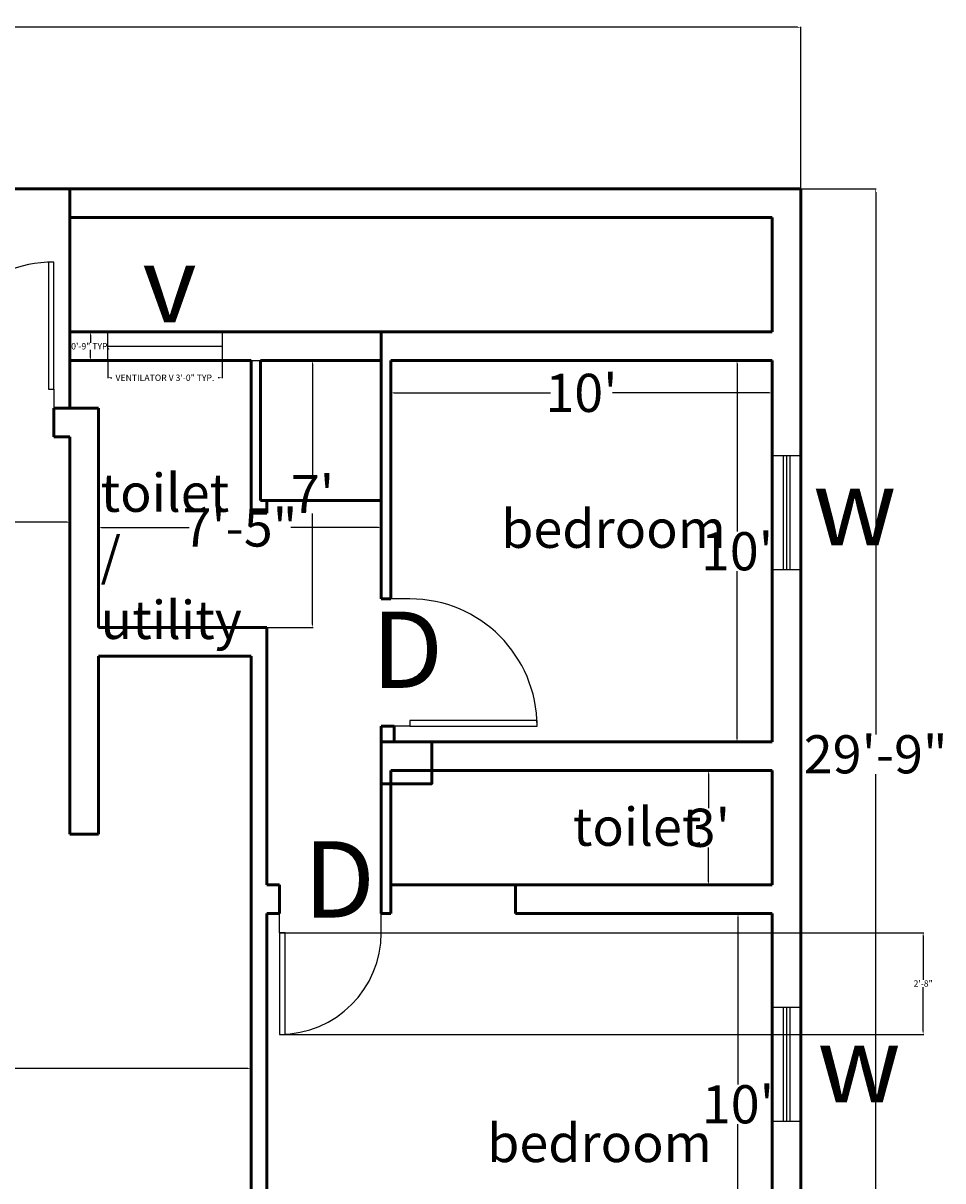
# Model space of a CAD drawing. Units: inches. Extents: x 409 to 7572, y 7 to 725.
# Tile 26 of 38: x 4623 to 4913, y 360 to 725. Entities that reach past the tile are written whole.
import ezdxf

# ---------------------------------------------------------------- set-up
doc = ezdxf.new("R2010")
doc.units = ezdxf.units.IN
doc.header["$MEASUREMENT"] = 0
for name, color, linetype, lineweight in [('A-ANNO-DIMS', 2, 'Continuous', 18), ('A-ANNO-SYMB', 3, 'Continuous', 25), ('A-AREA-IDEN', 7, 'Continuous', 25), ('A-DOOR', 3, 'Continuous', 25), ('A-GLAZ', 4, 'Continuous', 25), ('A-WALL', 7, 'Continuous', 50)]:
    doc.layers.add(name, color=color, linetype=linetype, lineweight=lineweight)
doc.styles.get("Standard").update_dxf_attribs({"font": 'arial.ttf'})
doc.dimstyles.get("Standard").update_dxf_attribs({"dimtxt": 2, "dimasz": 1, "dimexe": 0.18, "dimexo": 0.0625, "dimgap": 0.09, "dimtad": 0, "dimtih": 1, "dimtoh": 1, "dimdec": 0, "dimzin": 0, "dimdsep": 46, "dimlunit": 3, "dimtxsty": 'Standard', "dimcen": 0.09, "dimadec": 0, "dimazin": 0, "dimtfac": 1, "dimtdec": 0, "dimtofl": 0, "dimtmove": 0, "dimatfit": 3, "dimfxl": 1, "dimtolj": 1, "dimtzin": 0, "dimarcsym": 0})

# ---------------------------------------------------------------- blocks, each defined once
blk = doc.blocks.new('*U2')
for p, q in [((0, 0), (0, -6)), ((-40, 0), (-40, -6))]:
    blk.add_line(p, q)
blk.add_lwpolyline([(0, 0), (0, 40), (-1.75, 40), (-1.75, 0)], close=True)
blk.add_arc((0, 0), 40, 90, 180)
blk = doc.blocks.new('*U6')
for p, q in [((0, 0), (0, -6)), ((-40, 0), (-40, -6))]:
    blk.add_line(p, q)
blk.add_lwpolyline([(0, 0), (0, 40), (-1.75, 40), (-1.75, 0)], close=True)
blk.add_arc((0, 0), 40, 90, 180)
blk = doc.blocks.new('*U7')
for p, q in [((0, 0), (0, 6)), ((32, 0), (32, 6))]:
    blk.add_line(p, q)
blk.add_lwpolyline([(0, 0), (0, -32), (1.75, -32), (1.75, 0)], close=True)
blk.add_arc((0, 0), 32, 270, 0)
blk = doc.blocks.new('*D101')
at = {"layer": 'A-ANNO-DIMS', "color": 0, "lineweight": -2, "transparency": 16777216}
for p, q in [((4738.94, 618.47), (4738.94, 608.19)), ((4858.94, 618.47), (4858.94, 608.19)), ((4739.94, 608.37), (4789.23, 608.37)), ((4857.94, 608.37), (4808.65, 608.37))]:
    blk.add_line(p, q, dxfattribs=at)
at = {"layer": 'A-ANNO-DIMS', "color": 0, "transparency": 16777216}
for points in [[(4739.94, 608.54), (4739.94, 608.2), (4738.94, 608.37)], [(4857.94, 608.54), (4857.94, 608.2), (4858.94, 608.37)]]:
    blk.add_solid(points, dxfattribs=at)
at = {"layer": 'DEFPOINTS', "color": 0, "transparency": 16777216}
for p in [(4738.94, 618.53), (4858.94, 618.53), (4738.94, 608.37)]:
    blk.add_point(p, dxfattribs=at)
at = {"layer": 'A-ANNO-DIMS', "color": 0, "transparency": 16777216, "insert": (4798.94, 608.37), "char_height": 2, "attachment_point": 5}
blk.add_mtext("\\A1;{\\H6x;10'}", dxfattribs=at)
blk = doc.blocks.new('*D102')
at = {"layer": 'A-ANNO-DIMS', "color": 0, "lineweight": -2, "transparency": 16777216}
for p, q in [((4858.88, 618.53), (4847.71, 618.53)), ((4847.89, 617.53), (4847.89, 564.75)), ((4847.89, 499.53), (4847.89, 552.31)), ((4858.88, 498.53), (4847.71, 498.53))]:
    blk.add_line(p, q, dxfattribs=at)
at = {"layer": 'A-ANNO-DIMS', "color": 0, "transparency": 16777216}
for points in [[(4847.72, 617.53), (4848.06, 617.53), (4847.89, 618.53)], [(4847.72, 499.53), (4848.06, 499.53), (4847.89, 498.53)]]:
    blk.add_solid(points, dxfattribs=at)
at = {"layer": 'DEFPOINTS', "color": 0, "transparency": 16777216}
for p in [(4847.89, 618.53), (4858.94, 618.53), (4858.94, 498.53)]:
    blk.add_point(p, dxfattribs=at)
at = {"layer": 'A-ANNO-DIMS', "color": 0, "transparency": 16777216, "insert": (4847.89, 558.53), "char_height": 2, "attachment_point": 5}
blk.add_mtext("\\A1;{\\H6x;10'}", dxfattribs=at)
blk = doc.blocks.new('*D103')
at = {"layer": 'A-ANNO-DIMS', "color": 0, "lineweight": -2, "transparency": 16777216}
for p, q in [((4858.88, 444.53), (4848, 444.53)), ((4848.18, 443.53), (4848.18, 390.75)), ((4848.18, 325.53), (4848.18, 378.31)), ((4858.88, 324.53), (4848, 324.53))]:
    blk.add_line(p, q, dxfattribs=at)
at = {"layer": 'A-ANNO-DIMS', "color": 0, "transparency": 16777216}
for points in [[(4848.01, 443.53), (4848.34, 443.53), (4848.18, 444.53)], [(4848.01, 325.53), (4848.34, 325.53), (4848.18, 324.53)]]:
    blk.add_solid(points, dxfattribs=at)
at = {"layer": 'DEFPOINTS', "color": 0, "transparency": 16777216}
for p in [(4848.18, 444.53), (4858.94, 444.53), (4858.94, 324.53)]:
    blk.add_point(p, dxfattribs=at)
at = {"layer": 'A-ANNO-DIMS', "color": 0, "transparency": 16777216, "insert": (4848.18, 384.53), "char_height": 2, "attachment_point": 5}
blk.add_mtext("\\A1;{\\H6x;10'}", dxfattribs=at)
blk = doc.blocks.new('*D107')
at = {"layer": 'A-ANNO-DIMS', "color": 0, "lineweight": -2, "transparency": 16777216}
for p, q in [((4502.94, 563.4), (4502.94, 567.87)), ((4503.94, 567.69), (4550.3, 567.69)), ((4636.94, 567.69), (4590.58, 567.69)), ((4637.94, 563.4), (4637.94, 567.87))]:
    blk.add_line(p, q, dxfattribs=at)
at = {"layer": 'A-ANNO-DIMS', "color": 0, "transparency": 16777216}
for points in [[(4503.94, 567.86), (4503.94, 567.52), (4502.94, 567.69)], [(4636.94, 567.86), (4636.94, 567.52), (4637.94, 567.69)]]:
    blk.add_solid(points, dxfattribs=at)
at = {"layer": 'DEFPOINTS', "color": 0, "transparency": 16777216}
for p in [(4637.94, 567.69), (4502.94, 563.33), (4637.94, 563.33)]:
    blk.add_point(p, dxfattribs=at)
at = {"layer": 'A-ANNO-DIMS', "color": 0, "transparency": 16777216, "insert": (4570.44, 567.69), "char_height": 2, "attachment_point": 5}
blk.add_mtext('\\A1;{\\H6x;11\'-3"}', dxfattribs=at)
blk = doc.blocks.new('*D108')
at = {"layer": 'A-ANNO-DIMS', "color": 0, "lineweight": -2, "transparency": 16777216}
for p, q in [((4502.94, 403.47), (4502.94, 395.65)), ((4694.94, 403.47), (4694.94, 395.65)), ((4503.94, 395.83), (4589.23, 395.83)), ((4693.94, 395.83), (4608.65, 395.83))]:
    blk.add_line(p, q, dxfattribs=at)
at = {"layer": 'A-ANNO-DIMS', "color": 0, "transparency": 16777216}
for points in [[(4503.94, 396), (4503.94, 395.66), (4502.94, 395.83)], [(4693.94, 396), (4693.94, 395.66), (4694.94, 395.83)]]:
    blk.add_solid(points, dxfattribs=at)
at = {"layer": 'DEFPOINTS', "color": 0, "transparency": 16777216}
for p in [(4502.94, 403.53), (4694.94, 403.53), (4694.94, 395.83)]:
    blk.add_point(p, dxfattribs=at)
at = {"layer": 'A-ANNO-DIMS', "color": 0, "transparency": 16777216, "insert": (4598.94, 395.83), "char_height": 2, "attachment_point": 5}
blk.add_mtext("\\A1;{\\H6x;16'}", dxfattribs=at)
blk = doc.blocks.new('*D113')
at = {"layer": 'A-ANNO-DIMS', "color": 0, "lineweight": -2, "transparency": 16777216}
for p, q in [((4646.94, 568.97), (4646.94, 565.83)), ((4735.94, 568.97), (4735.94, 565.83)), ((4647.94, 566.01), (4675.45, 566.01)), ((4734.94, 566.01), (4707.43, 566.01))]:
    blk.add_line(p, q, dxfattribs=at)
at = {"layer": 'A-ANNO-DIMS', "color": 0, "transparency": 16777216}
for points in [[(4647.94, 566.17), (4647.94, 565.84), (4646.94, 566.01)], [(4734.94, 566.17), (4734.94, 565.84), (4735.94, 566.01)]]:
    blk.add_solid(points, dxfattribs=at)
at = {"layer": 'DEFPOINTS', "color": 0, "transparency": 16777216}
for p in [(4646.94, 569.03), (4735.94, 569.03), (4735.94, 566.01)]:
    blk.add_point(p, dxfattribs=at)
at = {"layer": 'A-ANNO-DIMS', "color": 0, "transparency": 16777216, "insert": (4691.44, 566.01), "char_height": 2, "attachment_point": 5}
blk.add_mtext('\\A1;{\\H6x;7\'-5"}', dxfattribs=at)
blk = doc.blocks.new('*D114')
at = {"layer": 'A-ANNO-DIMS', "color": 0, "lineweight": -2, "transparency": 16777216}
for p, q in [((4666.5, 618.53), (4714.48, 618.53)), ((4714.3, 617.53), (4714.3, 582.62)), ((4714.3, 535.53), (4714.3, 570.44)), ((4666.5, 534.53), (4714.48, 534.53))]:
    blk.add_line(p, q, dxfattribs=at)
at = {"layer": 'A-ANNO-DIMS', "color": 0, "transparency": 16777216}
for points in [[(4714.13, 617.53), (4714.47, 617.53), (4714.3, 618.53)], [(4714.13, 535.53), (4714.47, 535.53), (4714.3, 534.53)]]:
    blk.add_solid(points, dxfattribs=at)
at = {"layer": 'DEFPOINTS', "color": 0, "transparency": 16777216}
for p in [(4666.44, 618.53), (4666.44, 534.53), (4714.3, 534.53)]:
    blk.add_point(p, dxfattribs=at)
at = {"layer": 'A-ANNO-DIMS', "color": 0, "transparency": 16777216, "insert": (4714.3, 576.53), "char_height": 2, "attachment_point": 5}
blk.add_mtext("\\A1;{\\H6x;7'}", dxfattribs=at)
blk = doc.blocks.new('*D116')
at = {"layer": 'A-ANNO-DIMS', "color": 0, "lineweight": -2, "transparency": 16777216}
for p, q in [((4858.88, 489.53), (4838.69, 489.53)), ((4838.87, 488.53), (4838.87, 477.75)), ((4838.87, 454.53), (4838.87, 465.31)), ((4858.88, 453.53), (4838.69, 453.53))]:
    blk.add_line(p, q, dxfattribs=at)
at = {"layer": 'A-ANNO-DIMS', "color": 0, "transparency": 16777216}
for points in [[(4838.7, 488.53), (4839.03, 488.53), (4838.87, 489.53)], [(4838.7, 454.53), (4839.03, 454.53), (4838.87, 453.53)]]:
    blk.add_solid(points, dxfattribs=at)
at = {"layer": 'DEFPOINTS', "color": 0, "transparency": 16777216}
for p in [(4858.94, 489.53), (4838.87, 453.53), (4858.94, 453.53)]:
    blk.add_point(p, dxfattribs=at)
at = {"layer": 'A-ANNO-DIMS', "color": 0, "transparency": 16777216, "insert": (4838.87, 471.53), "char_height": 2, "attachment_point": 5}
blk.add_mtext("\\A1;{\\H6x;3'}", dxfattribs=at)
blk = doc.blocks.new('*D118')
at = {"layer": 'A-ANNO-DIMS', "color": 0, "lineweight": -2, "transparency": 16777216}
for p, q in [((4325.94, 672.59), (4325.94, 723.56)), ((4326.94, 723.38), (4593.38, 723.38)), ((4866.94, 723.38), (4600.51, 723.38)), ((4867.94, 672.59), (4867.94, 723.56))]:
    blk.add_line(p, q, dxfattribs=at)
at = {"layer": 'A-ANNO-DIMS', "color": 0, "transparency": 16777216}
for points in [[(4326.94, 723.55), (4326.94, 723.22), (4325.94, 723.38)], [(4866.94, 723.55), (4866.94, 723.22), (4867.94, 723.38)]]:
    blk.add_solid(points, dxfattribs=at)
at = {"layer": 'DEFPOINTS', "color": 0, "transparency": 16777216}
for p in [(4325.94, 723.38), (4325.94, 672.53), (4867.94, 672.53)]:
    blk.add_point(p, dxfattribs=at)
at = {"layer": 'A-ANNO-DIMS', "color": 0, "transparency": 16777216, "insert": (4596.94, 723.38), "char_height": 2, "attachment_point": 5}
blk.add_mtext('\\A1;45\'-2"', dxfattribs=at)
blk = doc.blocks.new('*D120')
at = {"layer": 'A-ANNO-DIMS', "color": 0, "lineweight": -2, "transparency": 16777216}
for p, q in [((4868, 672.53), (4891.69, 672.53)), ((4891.51, 671.53), (4891.51, 500.86)), ((4891.51, 316.53), (4891.51, 488.43)), ((4868, 315.53), (4891.69, 315.53))]:
    blk.add_line(p, q, dxfattribs=at)
at = {"layer": 'A-ANNO-DIMS', "color": 0, "transparency": 16777216}
for points in [[(4891.34, 671.53), (4891.67, 671.53), (4891.51, 672.53)], [(4891.34, 316.53), (4891.67, 316.53), (4891.51, 315.53)]]:
    blk.add_solid(points, dxfattribs=at)
at = {"layer": 'DEFPOINTS', "color": 0, "transparency": 16777216}
for p in [(4867.94, 672.53), (4891.51, 672.53), (4867.94, 315.53)]:
    blk.add_point(p, dxfattribs=at)
at = {"layer": 'A-ANNO-DIMS', "color": 0, "transparency": 16777216, "insert": (4891.51, 494.65), "char_height": 2, "attachment_point": 5}
blk.add_mtext('\\A1;{\\H6x;29\'-9"}', dxfattribs=at)
blk = doc.blocks.new('WIN-36')
for p, q in [((1699.82, 514.65), (1699.82, 478.65)), ((1700.82, 514.65), (1700.82, 478.65)), ((1701.82, 514.65), (1701.82, 478.65))]:
    blk.add_line(p, q)
blk.add_lwpolyline([(1705.32, 514.65), (1705.32, 478.65), (1696.32, 478.65), (1696.32, 514.65)], close=True)
blk = doc.blocks.new('VENT-36')
blk.add_line((5633.28, 355.73), (5633.28, 391.73))
blk.add_lwpolyline([(5628.78, 355.73), (5628.78, 391.73), (5637.78, 391.73), (5637.78, 355.73)], close=True)
blk = doc.blocks.new('*D169')
at = {"layer": 'A-ANNO-DIMS', "color": 0, "lineweight": -2, "transparency": 16777216}
for p, q in [((4649.86, 618.47), (4649.86, 612.95)), ((4685.86, 618.47), (4685.86, 612.95)), ((4650.86, 613.13), (4651.14, 613.13)), ((4684.86, 613.13), (4684.57, 613.13))]:
    blk.add_line(p, q, dxfattribs=at)
at = {"layer": 'A-ANNO-DIMS', "color": 0, "transparency": 16777216}
for points in [[(4650.86, 613.3), (4650.86, 612.96), (4649.86, 613.13)], [(4684.86, 613.3), (4684.86, 612.96), (4685.86, 613.13)]]:
    blk.add_solid(points, dxfattribs=at)
at = {"layer": 'DEFPOINTS', "color": 0, "transparency": 16777216}
for p in [(4649.86, 618.53), (4685.86, 618.53), (4685.86, 613.13)]:
    blk.add_point(p, dxfattribs=at)
at = {"layer": 'A-ANNO-DIMS', "color": 0, "transparency": 16777216, "insert": (4667.86, 613.13), "char_height": 2, "attachment_point": 5}
blk.add_mtext('\\A1;VENTILATOR V 3\'-0" TYP.', dxfattribs=at)
blk = doc.blocks.new('*D170')
at = {"layer": 'A-ANNO-DIMS', "color": 0, "lineweight": -2, "transparency": 16777216}
for p, q in [((4649.79, 627.53), (4644.28, 627.53)), ((4644.46, 626.53), (4644.46, 624.14)), ((4644.46, 619.53), (4644.46, 621.92)), ((4649.79, 618.53), (4644.28, 618.53))]:
    blk.add_line(p, q, dxfattribs=at)
at = {"layer": 'A-ANNO-DIMS', "color": 0, "transparency": 16777216}
for points in [[(4644.29, 626.53), (4644.62, 626.53), (4644.46, 627.53)], [(4644.29, 619.53), (4644.62, 619.53), (4644.46, 618.53)]]:
    blk.add_solid(points, dxfattribs=at)
at = {"layer": 'DEFPOINTS', "color": 0, "transparency": 16777216}
for p in [(4649.86, 627.53), (4644.46, 618.53), (4649.86, 618.53)]:
    blk.add_point(p, dxfattribs=at)
at = {"layer": 'A-ANNO-DIMS', "color": 0, "transparency": 16777216, "insert": (4644.46, 623.03), "char_height": 2, "attachment_point": 5}
blk.add_mtext('\\A1;0\'-9" TYP.', dxfattribs=at)
blk = doc.blocks.new('*D190')
at = {"layer": 'A-ANNO-DIMS', "color": 0, "lineweight": -2, "transparency": 16777216}
for p, q in [((4704, 438.53), (4906.62, 438.53)), ((4906.44, 437.53), (4906.44, 423.64)), ((4906.44, 407.53), (4906.44, 421.42)), ((4704, 406.53), (4906.62, 406.53))]:
    blk.add_line(p, q, dxfattribs=at)
at = {"layer": 'A-ANNO-DIMS', "color": 0, "transparency": 16777216}
for points in [[(4906.27, 437.53), (4906.61, 437.53), (4906.44, 438.53)], [(4906.27, 407.53), (4906.61, 407.53), (4906.44, 406.53)]]:
    blk.add_solid(points, dxfattribs=at)
at = {"layer": 'DEFPOINTS', "color": 0, "transparency": 16777216}
for p in [(4703.94, 438.53), (4703.94, 406.53), (4906.44, 406.53)]:
    blk.add_point(p, dxfattribs=at)
at = {"layer": 'A-ANNO-DIMS', "color": 0, "transparency": 16777216, "insert": (4906.44, 422.53), "char_height": 2, "attachment_point": 5}
blk.add_mtext('\\A1;2\'-8"', dxfattribs=at)

msp = doc.modelspace()

# ---------------------------------------------------------------- linework, layer by layer
at = {"layer": 'A-WALL'}
for p, q in [((4867.94, 672.53), (4325.94, 672.53)), ((4637.94, 672.53), (4637.94, 603.53)), ((4867.94, 315.53), (4867.94, 672.53)), ((4858.94, 663.53), (4637.94, 663.53)), ((4858.94, 627.53), (4858.94, 663.53)), ((4858.94, 627.53), (4637.94, 627.53)), ((4735.94, 627.53), (4735.94, 543.53)), ((4694.94, 618.53), (4637.94, 618.53)), ((4694.94, 618.53), (4694.94, 570.53)), ((4735.94, 618.53), (4697.94, 618.53)), ((4697.94, 618.53), (4697.94, 574.53)), ((4858.94, 618.53), (4738.94, 618.53)), ((4738.94, 618.53), (4738.94, 543.53)), ((4858.94, 498.53), (4858.94, 618.53)), ((4632.94, 603.53), (4646.94, 603.53)), ((4632.94, 603.53), (4632.94, 594.53)), ((4646.94, 603.53), (4646.94, 534.53)), ((4632.94, 594.53), (4637.94, 594.53)), ((4735.94, 574.53), (4697.94, 574.53)), ((4699.94, 574.53), (4699.94, 570.53)), ((4699.94, 570.53), (4694.94, 570.53)), ((4738.94, 543.53), (4735.94, 543.53)), ((4699.94, 534.53), (4646.94, 534.53)), ((4699.94, 534.53), (4699.94, 453.53)), ((4694.94, 525.53), (4646.94, 525.53)), ((4646.94, 525.53), (4646.94, 469.53)), ((4694.94, 525.53), (4694.94, 337.53)), ((4735.94, 498.53), (4735.94, 503.53)), ((4735.94, 503.53), (4739.94, 503.53)), ((4739.94, 503.53), (4739.94, 498.53)), ((4858.94, 498.53), (4735.94, 498.53)), ((4735.94, 498.53), (4735.94, 444.53)), ((4694.94, 489.53), (4694.94, 337.53)), ((4858.94, 489.53), (4738.94, 489.53)), ((4738.94, 489.53), (4738.94, 444.53)), ((4858.94, 453.53), (4858.94, 489.53)), ((4637.94, 469.53), (4646.94, 469.53)), ((4703.94, 453.53), (4699.94, 453.53)), ((4703.94, 453.53), (4703.94, 444.53)), ((4858.94, 453.53), (4738.94, 453.53)), ((4778.13, 453.53), (4778.13, 444.53)), ((4703.94, 444.53), (4699.94, 444.53)), ((4699.94, 444.53), (4699.94, 324.53)), ((4738.94, 444.53), (4735.94, 444.53)), ((4738.94, 444.53), (4735.94, 444.53)), ((4858.94, 444.53), (4778.13, 444.53)), ((4858.94, 324.53), (4858.94, 444.53))]:
    msp.add_line(p, q, dxfattribs=at)
msp.add_lwpolyline([(4637.94, 594.53), (4637.94, 525.53), (4637.94, 469.53)], dxfattribs=at)
msp.add_lwpolyline([(4735.94, 498.53), (4751.81, 498.53), (4751.81, 485.36), (4735.94, 485.36)], close=True, dxfattribs=at)

# ---------------------------------------------------------------- block references
at = {"layer": 'A-DOOR'}
for name, p in [('*U2', (4632.94, 609.53)), ('*U7', (4703.94, 438.53))]:
    msp.add_blockref(name, p, dxfattribs=at)
at = {"layer": 'A-DOOR', "rotation": 270}
msp.add_blockref('*U6', (4744.94, 503.53), dxfattribs=at)
at = {"layer": 'A-GLAZ', "rotation": 269.9999999999999}
msp.add_blockref('VENT-36', (4294.13, 6256.31), dxfattribs=at)
at = {"layer": 'A-GLAZ'}
for p in [(3162.62, 73.99), (3162.62, -99.57)]:
    msp.add_blockref('WIN-36', p, dxfattribs=at)

# ---------------------------------------------------------------- texts
at = {"layer": 'A-ANNO-SYMB', "char_height": 24, "attachment_point": 1}
for s, width, insert in [('v', 18.2582, (4660.77, 654.6)), ('w', 18.2582, (4871.77, 584.43)), ('D', 19.1972, (4732.87, 539.54)), ('D', 19.1972, (4711.44, 467.28)), ('w', 18.2582, (4873.14, 409.16))]:
    msp.add_mtext_dynamic_manual_height_columns(s, width=width, gutter_width=1, heights=[0], dxfattribs=dict(at, insert=insert))
at = {"layer": 'A-AREA-IDEN', "char_height": 12, "attachment_point": 1}
for s, width, insert in [('toilet / utility', 49.2946, (4647.59, 582.94)), ('bedroom', 40.9017, (4773.69, 571.6)), ('toilet', 49.2946, (4796.19, 477.86)), ('bedroom', 40.9017, (4769.27, 378.34))]:
    msp.add_mtext_dynamic_manual_height_columns(s, width=width, gutter_width=1, heights=[0], dxfattribs=dict(at, insert=insert))

# ---------------------------------------------------------------- dimensions: what is measured, and where the dimension line sits
at = {"layer": 'A-ANNO-DIMS'}
dim = msp.add_linear_dim(base=(4325.94, 723.38), p1=(4867.94, 672.53), p2=(4325.94, 672.53), dimstyle='Standard', override={"dimclrd": 0, "dimclre": 0, "dimclrt": 0}, dxfattribs=at)
dim.commit()
dim.dimension.update_dxf_attribs({"geometry": '*D118', "text_midpoint": (4596.94, 723.38)})
dim = msp.add_linear_dim(base=(4891.51, 672.53), p1=(4867.94, 315.53), p2=(4867.94, 672.53), angle=90, text='{\\H6x;<>}', dimstyle='Standard', override={"dimclrd": 0, "dimclre": 0, "dimclrt": 0}, dxfattribs=at)
dim.commit()
dim.dimension.update_dxf_attribs({"geometry": '*D120', "text_midpoint": (4891.51, 494.65), "dimtype": 160})
for base, p1, p2, angle, text, override, picture, middle in [((4644.46, 618.53), (4649.86, 627.53), (4649.86, 618.53), 270, '<> TYP.', {"dimdec": 1, "dimrnd": 0, "dimzin": 1, "dimlunit": 4, "dimfrac": 2}, '*D170', (4644.46, 623.03)), ((4714.3, 534.53), (4666.44, 618.53), (4666.44, 534.53), 90, '{\\H6x;<>}', {"dimclrd": 0, "dimclre": 0, "dimclrt": 0}, '*D114', (4714.3, 576.53)), ((4847.89, 618.53), (4858.94, 498.53), (4858.94, 618.53), 90, '{\\H6x;<>}', {"dimclrd": 0, "dimclre": 0, "dimclrt": 0}, '*D102', (4847.89, 558.53)), ((4838.87, 453.53), (4858.94, 489.53), (4858.94, 453.53), 90, '{\\H6x;<>}', {"dimclrd": 0, "dimclre": 0, "dimclrt": 0}, '*D116', (4838.87, 471.53)), ((4848.18, 444.53), (4858.94, 324.53), (4858.94, 444.53), 90, '{\\H6x;<>}', {"dimclrd": 0, "dimclre": 0, "dimclrt": 0}, '*D103', (4848.18, 384.53))]:
    dim = msp.add_linear_dim(base=base, p1=p1, p2=p2, angle=angle, text=text, dimstyle='Standard', override=override, dxfattribs=at)
    dim.commit()
    dim.dimension.update_dxf_attribs({"geometry": picture, "text_midpoint": middle})
for base, p1, p2, text, override, picture, middle in [((4685.86, 613.13), (4649.86, 618.53), (4685.86, 618.53), 'VENTILATOR V <> TYP.', {"dimdec": 1, "dimrnd": 0, "dimzin": 1, "dimlunit": 4, "dimfrac": 2}, '*D169', (4667.86, 613.13)), ((4738.94, 608.37), (4858.94, 618.53), (4738.94, 618.53), '{\\H6x;<>}', {"dimclrd": 0, "dimclre": 0, "dimclrt": 0}, '*D101', (4798.94, 608.37)), ((4637.94, 567.69), (4502.94, 563.33), (4637.94, 563.33), '{\\H6x;<>}', {"dimclrd": 0, "dimclre": 0, "dimclrt": 0}, '*D107', (4570.44, 567.69)), ((4735.94, 566.01), (4646.94, 569.03), (4735.94, 569.03), '{\\H6x;<>}', {"dimclrd": 0, "dimclre": 0, "dimclrt": 0}, '*D113', (4691.44, 566.01))]:
    dim = msp.add_linear_dim(base=base, p1=p1, p2=p2, text=text, dimstyle='Standard', override=override, dxfattribs=at)
    dim.commit()
    dim.dimension.update_dxf_attribs({"geometry": picture, "text_midpoint": middle})
dim = msp.add_linear_dim(base=(4906.44, 406.53), p1=(4703.94, 438.53), p2=(4703.94, 406.53), angle=90, dimstyle='Standard', override={"dimdec": 1, "dimlfac": 1, "dimrnd": 0, "dimzin": 1, "dimdsep": 46, "dimlunit": 4, "dimfrac": 2}, dxfattribs=at)
dim.commit()
dim.dimension.update_dxf_attribs({"geometry": '*D190', "text_midpoint": (4906.44, 422.53)})
dim = msp.add_linear_dim(base=(4694.94, 395.83), p1=(4502.94, 403.53), p2=(4694.94, 403.53), text='{\\H6x;<>}', dimstyle='Standard', override={"dimclrd": 0, "dimclre": 0, "dimclrt": 0}, dxfattribs=at)
dim.commit()
dim.dimension.update_dxf_attribs({"geometry": '*D108', "text_midpoint": (4598.94, 395.83), "dimtype": 160})

doc.saveas('drawing.dxf')
